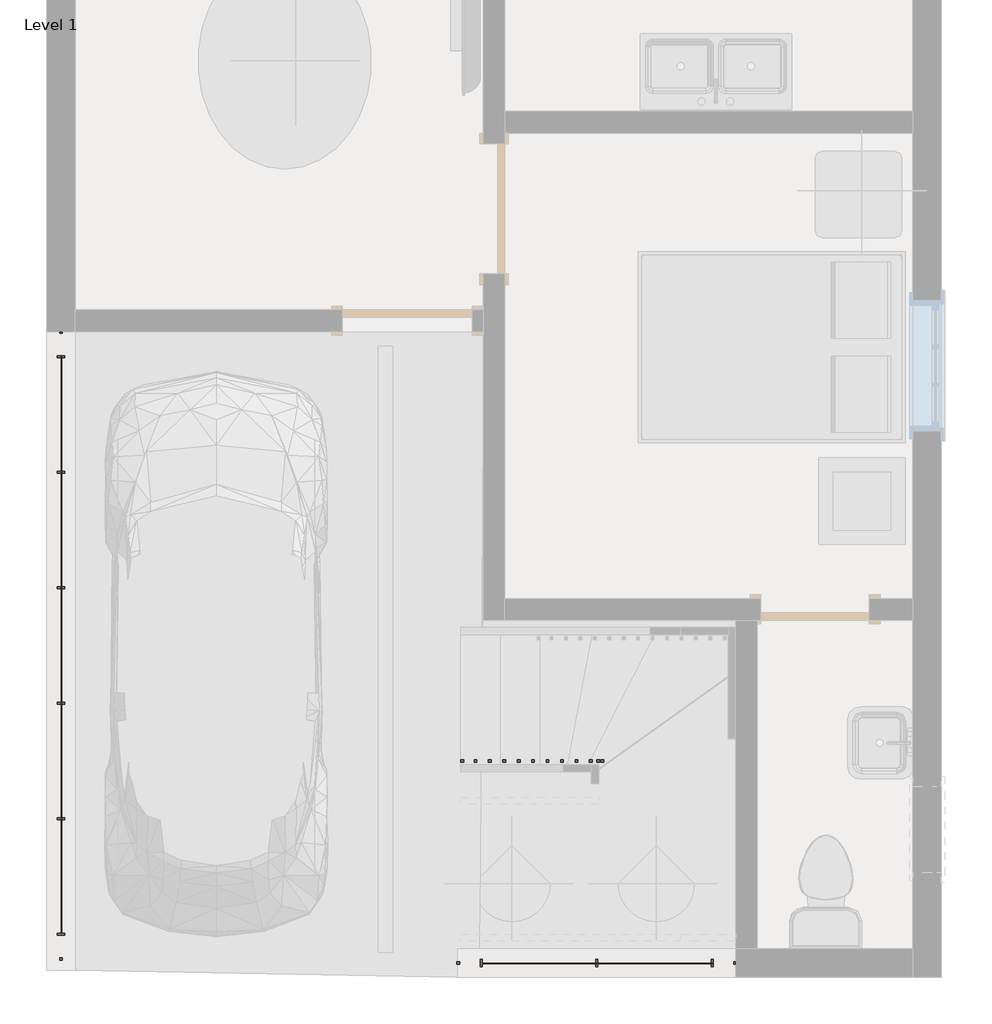
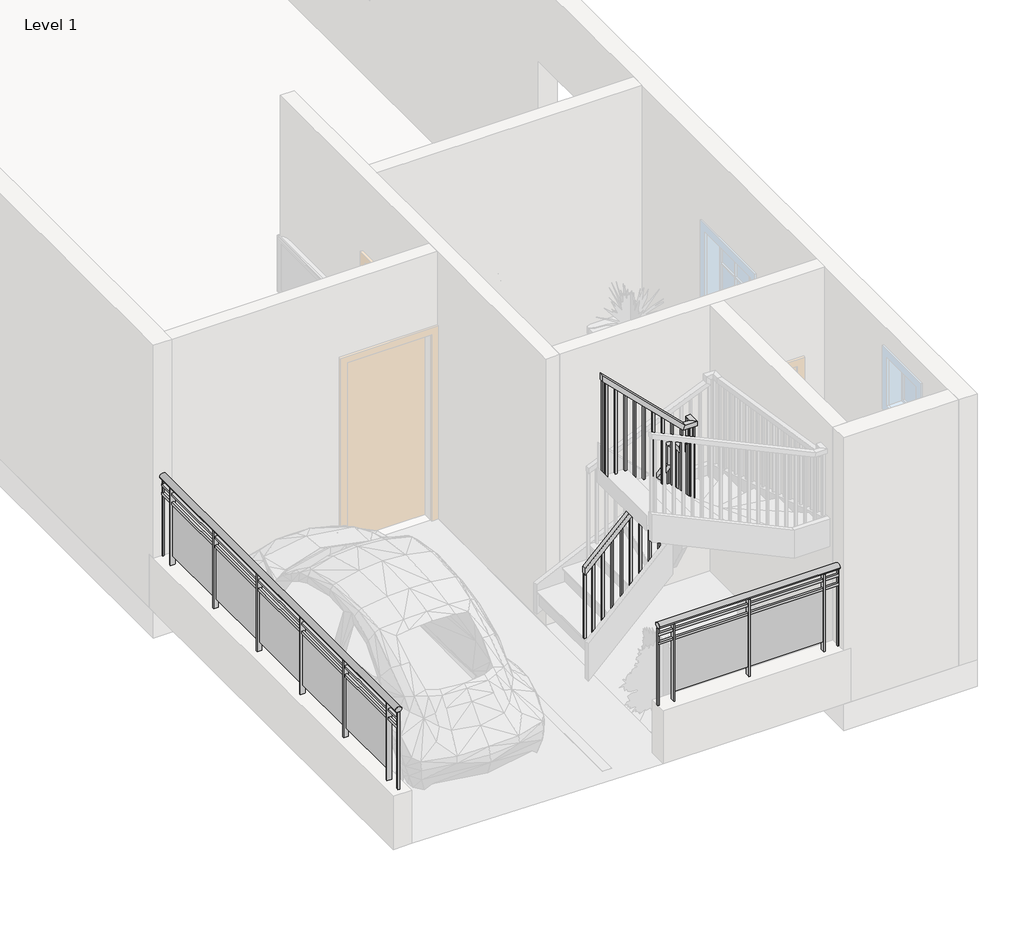
# One storey, part 2 of 3: 3 railings.
"""IFC4 building model written with IfcOpenShell, lengths in millimetres."""

from ifc_helpers import new_model, si_unit, point, frame, origin, place, context, project, spatial, polyline, ellipse_curve, trimmed, outline, extrude, faceted_brep, element, save
from ifc_brep_helpers import plane_surface, extruded_surface, advanced_brep

model = new_model("IFC4")

# Units and contexts
model_context = context("Model", 3, world=origin())
ifc_project = project(units=[si_unit("LENGTHUNIT", "METRE", prefix="MILLI")], contexts=[model_context])

# Site, building, storey
site = spatial("IfcSite", under=ifc_project)
building = spatial("IfcBuilding", under=site)
storey = spatial("IfcBuildingStorey", under=building, Name="Level 1", Elevation=0.0)

# Railings
placement = place(None, origin())
element("IfcRailing", 1, ObjectType="Glass Panel - Bottom Fill", at=placement, inside=storey, context=model_context, shape_type="SolidModel", body=[
    advanced_brep(
    [(-14578.2112155, 1512.0104001, 1524.0), (-14654.4112155, 1512.0104001, 1524.0), (-14578.2112155, -2907.5895999, 1524.0), (-14654.4112155, -2907.5895999, 1524.0)],
    [
        (0, 1, ellipse_curve(frame((-14616.3112155, 1512.0104001, 1524.0), z_axis=(0.0, 1.0, 0.0), x_axis=(-1.0, 0.0, 0.0)), 38.1, 28.575)),
        (1, 0, ellipse_curve(frame((-14616.3112155, 1512.0104001, 1524.0), z_axis=(0.0, 1.0, 0.0), x_axis=(-1.0, 0.0, 0.0)), 38.1, 28.575)),
        (2, 3, ellipse_curve(frame((-14616.3112155, -2907.5895999, 1524.0), z_axis=(0.0, -1.0, 0.0), x_axis=(-1.0, 0.0, 0.0)), 38.1, 28.575)),
        (3, 2, ellipse_curve(frame((-14616.3112155, -2907.5895999, 1524.0), z_axis=(0.0, -1.0, 0.0), x_axis=(-1.0, 0.0, 0.0)), 38.1, 28.575)),
        (0, 2),
        (3, 1),
    ],
    [
        plane_surface(frame((-14616.3112155, 1512.0104001, 1524.0), z_axis=(0.0, 1.0, 0.0), x_axis=(0.0, 0.0, -1.0))),
        plane_surface(frame((-14616.3112155, -2907.5895999, 1524.0), z_axis=(0.0, -1.0, 0.0), x_axis=(0.0, 0.0, -1.0))),
        extruded_surface(trimmed(ellipse_curve(frame((-14616.3112155, -2907.5895999, 1524.0), z_axis=(0.0, 1.0, 0.0), x_axis=(-1.0, 0.0, 0.0)), 38.1, 28.575), [point((-14578.2112155, -2907.5895999, 1524.0))], [point((-14654.4112155, -2907.5895999, 1524.0))], True, "CARTESIAN"), (0.0, 4419.6, 0.0), 4419.6),
        extruded_surface(trimmed(ellipse_curve(frame((-14616.3112155, -2907.5895999, 1524.0), z_axis=(0.0, 1.0, 0.0), x_axis=(-1.0, 0.0, 0.0)), 38.1, 28.575), [point((-14654.4112155, -2907.5895999, 1524.0))], [point((-14578.2112155, -2907.5895999, 1524.0))], True, "CARTESIAN"), (0.0, 4419.6, 0.0), 4419.6),
    ],
    [
        (0, [[1, 2]]),
        (1, [[3, 4]]),
        (2, [[-1, 5, -4, 6]]),
        (3, [[-2, -6, -3, -5]]),
    ],
),
    extrude(outline(polyline([(-14629.0112155, 1512.0104001), (-14603.6112155, 1512.0104001), (-14603.6112155, -2907.5895999), (-14629.0112155, -2907.5895999), (-14629.0112155, 1512.0104001)])), frame((0.0, 0.0, 1409.7), z_axis=(0.0, 0.0, 1.0), x_axis=(1.0, 0.0, 0.0)), (0.0, 0.0, 1.0), 25.4),
    extrude(outline(polyline([(-14629.0112155, 1512.0104001), (-14603.6112155, 1512.0104001), (-14603.6112155, -2907.5895999), (-14629.0112155, -2907.5895999), (-14629.0112155, 1512.0104001)])), frame((0.0, 0.0, 1308.1), z_axis=(0.0, 0.0, 1.0), x_axis=(1.0, 0.0, 0.0)), (0.0, 0.0, 1.0), 25.4),
    extrude(outline(polyline([(-14641.7112155, -2723.4395999), (-14590.9112155, -2723.4395999), (-14590.9112155, -2736.1395999), (-14641.7112155, -2736.1395999), (-14641.7112155, -2723.4395999)])), frame((0.0, 0.0, 609.6), z_axis=(0.0, 0.0, 1.0), x_axis=(1.0, 0.0, 0.0)), (0.0, 0.0, 1.0), 885.6788223),
    extrude(outline(polyline([(-14609.7760585, -1916.9895999), (-14609.7760585, -2729.7895999), (-14616.1260585, -2729.7895999), (-14616.1260585, -1916.9895999), (-14609.7760585, -1916.9895999)])), frame((0.0, 0.0, 711.2), z_axis=(0.0, 0.0, 1.0), x_axis=(1.0, 0.0, 0.0)), (0.0, 0.0, 1.0), 596.9),
    extrude(outline(polyline([(-14641.7112155, -1910.6395999), (-14590.9112155, -1910.6395999), (-14590.9112155, -1923.3395999), (-14641.7112155, -1923.3395999), (-14641.7112155, -1910.6395999)])), frame((0.0, 0.0, 609.6), z_axis=(0.0, 0.0, 1.0), x_axis=(1.0, 0.0, 0.0)), (0.0, 0.0, 1.0), 885.6788223),
    extrude(outline(polyline([(-14609.7760585, -1104.1895999), (-14609.7760585, -1916.9895999), (-14616.1260585, -1916.9895999), (-14616.1260585, -1104.1895999), (-14609.7760585, -1104.1895999)])), frame((0.0, 0.0, 711.2), z_axis=(0.0, 0.0, 1.0), x_axis=(1.0, 0.0, 0.0)), (0.0, 0.0, 1.0), 596.9),
    extrude(outline(polyline([(-14641.7112155, -1097.8395999), (-14590.9112155, -1097.8395999), (-14590.9112155, -1110.5395999), (-14641.7112155, -1110.5395999), (-14641.7112155, -1097.8395999)])), frame((0.0, 0.0, 609.6), z_axis=(0.0, 0.0, 1.0), x_axis=(1.0, 0.0, 0.0)), (0.0, 0.0, 1.0), 885.6788223),
    extrude(outline(polyline([(-14609.7760585, -291.3895999), (-14609.7760585, -1104.1895999), (-14616.1260585, -1104.1895999), (-14616.1260585, -291.3895999), (-14609.7760585, -291.3895999)])), frame((0.0, 0.0, 711.2), z_axis=(0.0, 0.0, 1.0), x_axis=(1.0, 0.0, 0.0)), (0.0, 0.0, 1.0), 596.9),
    extrude(outline(polyline([(-14641.7112155, -285.0395999), (-14590.9112155, -285.0395999), (-14590.9112155, -297.7395999), (-14641.7112155, -297.7395999), (-14641.7112155, -285.0395999)])), frame((0.0, 0.0, 609.6), z_axis=(0.0, 0.0, 1.0), x_axis=(1.0, 0.0, 0.0)), (0.0, 0.0, 1.0), 885.6788223),
    extrude(outline(polyline([(-14609.7760585, 521.4104001), (-14609.7760585, -291.3895999), (-14616.1260585, -291.3895999), (-14616.1260585, 521.4104001), (-14609.7760585, 521.4104001)])), frame((0.0, 0.0, 711.2), z_axis=(0.0, 0.0, 1.0), x_axis=(1.0, 0.0, 0.0)), (0.0, 0.0, 1.0), 596.9),
    extrude(outline(polyline([(-14641.7112155, 527.7604001), (-14590.9112155, 527.7604001), (-14590.9112155, 515.0604001), (-14641.7112155, 515.0604001), (-14641.7112155, 527.7604001)])), frame((0.0, 0.0, 609.6), z_axis=(0.0, 0.0, 1.0), x_axis=(1.0, 0.0, 0.0)), (0.0, 0.0, 1.0), 885.6788223),
    extrude(outline(polyline([(-14609.7760585, 1334.2104001), (-14609.7760585, 521.4104001), (-14616.1260585, 521.4104001), (-14616.1260585, 1334.2104001), (-14609.7760585, 1334.2104001)])), frame((0.0, 0.0, 711.2), z_axis=(0.0, 0.0, 1.0), x_axis=(1.0, 0.0, 0.0)), (0.0, 0.0, 1.0), 596.9),
    extrude(outline(polyline([(-14641.7112155, 1340.5604001), (-14590.9112155, 1340.5604001), (-14590.9112155, 1327.8604001), (-14641.7112155, 1327.8604001), (-14641.7112155, 1340.5604001)])), frame((0.0, 0.0, 609.6), z_axis=(0.0, 0.0, 1.0), x_axis=(1.0, 0.0, 0.0)), (0.0, 0.0, 1.0), 885.6788223),
    extrude(outline(polyline([(-14625.8362155, -2894.8895999), (-14606.7862155, -2894.8895999), (-14606.7862155, -2913.9395999), (-14625.8362155, -2913.9395999), (-14625.8362155, -2894.8895999)])), frame((0.0, 0.0, 609.6), z_axis=(0.0, 0.0, 1.0), x_axis=(1.0, 0.0, 0.0)), (0.0, 0.0, 1.0), 885.6788223),
    extrude(outline(polyline([(-14625.8362155, 1518.3604001), (-14606.7862155, 1518.3604001), (-14606.7862155, 1499.3104001), (-14625.8362155, 1499.3104001), (-14625.8362155, 1518.3604001)])), frame((0.0, 0.0, 609.6), z_axis=(0.0, 0.0, 1.0), x_axis=(1.0, 0.0, 0.0)), (0.0, 0.0, 1.0), 885.6788223),
])
element("IfcRailing", 2, ObjectType="Glass Panel - Bottom Fill", at=placement, inside=storey, context=model_context, shape_type="SolidModel", body=[
    advanced_brep(
    [(-9866.5112155, -2971.0895999, 1524.0), (-9866.5112155, -2894.8895999, 1524.0), (-11822.3112155, -2971.0895999, 1524.0), (-11822.3112155, -2894.8895999, 1524.0)],
    [
        (0, 1, ellipse_curve(frame((-9866.5112155, -2932.9895999, 1524.0), z_axis=(1.0, 0.0, 0.0), x_axis=(0.0, 1.0, 0.0)), 38.1, 28.575)),
        (1, 0, ellipse_curve(frame((-9866.5112155, -2932.9895999, 1524.0), z_axis=(1.0, 0.0, 0.0), x_axis=(0.0, 1.0, 0.0)), 38.1, 28.575)),
        (2, 3, ellipse_curve(frame((-11822.3112155, -2932.9895999, 1524.0), z_axis=(-1.0, 0.0, 0.0), x_axis=(0.0, 1.0, 0.0)), 38.1, 28.575)),
        (3, 2, ellipse_curve(frame((-11822.3112155, -2932.9895999, 1524.0), z_axis=(-1.0, 0.0, 0.0), x_axis=(0.0, 1.0, 0.0)), 38.1, 28.575)),
        (0, 2),
        (3, 1),
    ],
    [
        plane_surface(frame((-9866.5112155, -2932.9895999, 1524.0), z_axis=(1.0, 0.0, 0.0), x_axis=(0.0, -1.0, 0.0))),
        plane_surface(frame((-11822.3112155, -2932.9895999, 1524.0), z_axis=(-1.0, 0.0, 0.0), x_axis=(0.0, -1.0, 0.0))),
        extruded_surface(trimmed(ellipse_curve(frame((-11822.3112155, -2932.9895999, 1524.0), z_axis=(1.0, 0.0, 0.0), x_axis=(0.0, 1.0, 0.0)), 38.1, 28.575), [point((-11822.3112155, -2971.0895999, 1524.0))], [point((-11822.3112155, -2894.8895999, 1524.0))], True, "CARTESIAN"), (1955.7999999999993, 0.0, 0.0), 1955.7999999999993),
        extruded_surface(trimmed(ellipse_curve(frame((-11822.3112155, -2932.9895999, 1524.0), z_axis=(1.0, 0.0, 0.0), x_axis=(0.0, 1.0, 0.0)), 38.1, 28.575), [point((-11822.3112155, -2894.8895999, 1524.0))], [point((-11822.3112155, -2971.0895999, 1524.0))], True, "CARTESIAN"), (1955.7999999999993, 0.0, 0.0), 1955.7999999999993),
    ],
    [
        (0, [[1, 2]]),
        (1, [[3, 4]]),
        (2, [[-1, 5, -4, 6]]),
        (3, [[-2, -6, -3, -5]]),
    ],
),
    extrude(outline(polyline([(-9866.5112155, -2920.2895999), (-9866.5112155, -2945.6895999), (-11822.3112155, -2945.6895999), (-11822.3112155, -2920.2895999), (-9866.5112155, -2920.2895999)])), frame((0.0, 0.0, 1409.7), z_axis=(0.0, 0.0, 1.0), x_axis=(1.0, 0.0, 0.0)), (0.0, 0.0, 1.0), 25.4),
    extrude(outline(polyline([(-9866.5112155, -2920.2895999), (-9866.5112155, -2945.6895999), (-11822.3112155, -2945.6895999), (-11822.3112155, -2920.2895999), (-9866.5112155, -2920.2895999)])), frame((0.0, 0.0, 1308.1), z_axis=(0.0, 0.0, 1.0), x_axis=(1.0, 0.0, 0.0)), (0.0, 0.0, 1.0), 25.4),
    extrude(outline(polyline([(-11650.8612155, -2907.5895999), (-11650.8612155, -2958.3895999), (-11663.5612155, -2958.3895999), (-11663.5612155, -2907.5895999), (-11650.8612155, -2907.5895999)])), frame((0.0, 0.0, 609.6), z_axis=(0.0, 0.0, 1.0), x_axis=(1.0, 0.0, 0.0)), (0.0, 0.0, 1.0), 885.6788223),
    extrude(outline(polyline([(-10844.4112155, -2939.5247569), (-11657.2112155, -2939.5247569), (-11657.2112155, -2933.1747569), (-10844.4112155, -2933.1747569), (-10844.4112155, -2939.5247569)])), frame((0.0, 0.0, 711.2), z_axis=(0.0, 0.0, 1.0), x_axis=(1.0, 0.0, 0.0)), (0.0, 0.0, 1.0), 596.9),
    extrude(outline(polyline([(-10838.0612155, -2907.5895999), (-10838.0612155, -2958.3895999), (-10850.7612155, -2958.3895999), (-10850.7612155, -2907.5895999), (-10838.0612155, -2907.5895999)])), frame((0.0, 0.0, 609.6), z_axis=(0.0, 0.0, 1.0), x_axis=(1.0, 0.0, 0.0)), (0.0, 0.0, 1.0), 885.6788223),
    extrude(outline(polyline([(-10031.6112155, -2939.5247569), (-10844.4112155, -2939.5247569), (-10844.4112155, -2933.1747569), (-10031.6112155, -2933.1747569), (-10031.6112155, -2939.5247569)])), frame((0.0, 0.0, 711.2), z_axis=(0.0, 0.0, 1.0), x_axis=(1.0, 0.0, 0.0)), (0.0, 0.0, 1.0), 596.9),
    extrude(outline(polyline([(-10025.2612155, -2907.5895999), (-10025.2612155, -2958.3895999), (-10037.9612155, -2958.3895999), (-10037.9612155, -2907.5895999), (-10025.2612155, -2907.5895999)])), frame((0.0, 0.0, 609.6), z_axis=(0.0, 0.0, 1.0), x_axis=(1.0, 0.0, 0.0)), (0.0, 0.0, 1.0), 885.6788223),
    extrude(outline(polyline([(-11809.6112155, -2923.4645999), (-11809.6112155, -2942.5145999), (-11828.6612155, -2942.5145999), (-11828.6612155, -2923.4645999), (-11809.6112155, -2923.4645999)])), frame((0.0, 0.0, 609.6), z_axis=(0.0, 0.0, 1.0), x_axis=(1.0, 0.0, 0.0)), (0.0, 0.0, 1.0), 885.6788223),
    extrude(outline(polyline([(-9860.1612155, -2923.4645999), (-9860.1612155, -2942.5145999), (-9879.2112155, -2942.5145999), (-9879.2112155, -2923.4645999), (-9860.1612155, -2923.4645999)])), frame((0.0, 0.0, 609.6), z_axis=(0.0, 0.0, 1.0), x_axis=(1.0, 0.0, 0.0)), (0.0, 0.0, 1.0), 885.6788223),
])
element("IfcRailing", 3, ObjectType="Handrail - Rectangular", at=placement, inside=storey, context=model_context, shape_type="SolidModel", body=[
    faceted_brep([(-11800.6429074, -1485.1895999, 1316.3704569), (-11800.6429074, -1485.1895999, 1245.0455517), (-11800.6429074, -1535.9895999, 1245.0455517), (-11800.6429074, -1535.9895999, 1316.3704569), (-10907.9112155, -1485.1895999, 2196.2028354), (-10857.1112155, -1485.1895999, 2174.9439077), (-10857.1112155, -1535.9895999, 2174.9439077), (-10907.9112155, -1535.9895999, 2196.2028354), (-10907.9112155, -1485.1895999, 2414.6281882), (-10857.1112155, -1485.1895999, 2363.8281882), (-10857.1112155, -1535.9895999, 2363.8281882), (-10907.9112155, -1535.9895999, 2414.6281882), (-10780.9112155, -1485.1895999, 2414.6281882), (-10780.9112155, -1485.1895999, 2363.8281882), (-10831.7112155, -1535.9895999, 2363.8281882), (-10831.7112155, -1535.9895999, 2414.6281882), (-10780.9112155, -1612.1895999, 2414.6281882), (-10780.9112155, -1641.3109337, 2363.8281882), (-10831.7112155, -1641.3109337, 2363.8281882), (-10831.7112155, -1612.1895999, 2414.6281882), (-10780.9112155, -1739.1895999, 2631.5051451), (-10780.9112155, -1789.9895999, 2617.7256424), (-10831.7112155, -1789.9895999, 2617.7256424), (-10831.7112155, -1739.1895999, 2631.5051451), (-10780.9112155, -1739.1895999, 2849.930498), (-10780.9112155, -1789.9895999, 2799.130498), (-10831.7112155, -1789.9895999, 2799.130498), (-10831.7112155, -1739.1895999, 2849.930498), (-10780.9112155, -1866.1895999, 2849.930498), (-10780.9112155, -1866.1895999, 2799.130498), (-10831.7112155, -1815.3895999, 2799.130498), (-10831.7112155, -1815.3895999, 2849.930498), (-10907.9112155, -1866.1895999, 2849.930498), (-10928.7370385, -1866.1895999, 2799.130498), (-10928.7370385, -1815.3895999, 2799.130498), (-10907.9112155, -1815.3895999, 2849.930498), (-11800.6429074, -1866.1895999, 3729.7628764), (-11800.6429074, -1815.3895999, 3729.7628764), (-11800.6429074, -1815.3895999, 3658.4379712), (-11800.6429074, -1866.1895999, 3658.4379712)], [[[0, 1, 2, 3]], [[1, 0, 4, 5]], [[2, 1, 5, 6]], [[3, 2, 6, 7]], [[0, 3, 7, 4]], [[5, 4, 8, 9]], [[6, 5, 9, 10]], [[7, 6, 10, 11]], [[4, 7, 11, 8]], [[9, 8, 12, 13]], [[10, 9, 13, 14]], [[11, 10, 14, 15]], [[8, 11, 15, 12]], [[13, 12, 16, 17]], [[14, 13, 17, 18]], [[15, 14, 18, 19]], [[12, 15, 19, 16]], [[17, 16, 20, 21]], [[18, 17, 21, 22]], [[19, 18, 22, 23]], [[16, 19, 23, 20]], [[21, 20, 24, 25]], [[22, 21, 25, 26]], [[23, 22, 26, 27]], [[20, 23, 27, 24]], [[25, 24, 28, 29]], [[26, 25, 29, 30]], [[27, 26, 30, 31]], [[24, 27, 31, 28]], [[29, 28, 32, 33]], [[30, 29, 33, 34]], [[31, 30, 34, 35]], [[28, 31, 35, 32]], [[36, 37, 38, 39]], [[33, 32, 36, 39]], [[34, 33, 39, 38]], [[35, 34, 38, 37]], [[32, 35, 37, 36]]]),
    extrude(outline(polyline([(3597.8779463, -11739.1950058), (3616.6526879, -11758.2450058), (2540.0, -11758.2450058), (2540.0, -11739.1950058), (3597.8779463, -11739.1950058)])), frame((0.0, -1850.3145999, 0.0), z_axis=(0.0, 1.0, 0.0), x_axis=(0.0, 0.0, 1.0)), (0.0, 0.0, 1.0), 19.05),
    extrude(outline(polyline([(3497.7459913, -11637.5950058), (3516.5207329, -11656.6450058), (2540.0, -11656.6450058), (2540.0, -11637.5950058), (3497.7459913, -11637.5950058)])), frame((0.0, -1850.3145999, 0.0), z_axis=(0.0, 1.0, 0.0), x_axis=(0.0, 0.0, 1.0)), (0.0, 0.0, 1.0), 19.05),
    extrude(outline(polyline([(3397.6140362, -11535.9950058), (3416.3887778, -11555.0450058), (2540.0, -11555.0450058), (2540.0, -11535.9950058), (3397.6140362, -11535.9950058)])), frame((0.0, -1850.3145999, 0.0), z_axis=(0.0, 1.0, 0.0), x_axis=(0.0, 0.0, 1.0)), (0.0, 0.0, 1.0), 19.05),
    extrude(outline(polyline([(3297.4820812, -11434.3950058), (3316.2568227, -11453.4450058), (2370.6666667, -11453.4450058), (2370.6666667, -11434.3950058), (3297.4820812, -11434.3950058)])), frame((0.0, -1850.3145999, 0.0), z_axis=(0.0, 1.0, 0.0), x_axis=(0.0, 0.0, 1.0)), (0.0, 0.0, 1.0), 19.05),
    extrude(outline(polyline([(3197.3501261, -11332.7950058), (3216.1248677, -11351.8450058), (2370.6666667, -11351.8450058), (2370.6666667, -11332.7950058), (3197.3501261, -11332.7950058)])), frame((0.0, -1850.3145999, 0.0), z_axis=(0.0, 1.0, 0.0), x_axis=(0.0, 0.0, 1.0)), (0.0, 0.0, 1.0), 19.05),
    extrude(outline(polyline([(3097.218171, -11231.1950058), (3115.9929126, -11250.2450058), (2201.3333333, -11250.2450058), (2201.3333333, -11231.1950058), (3097.218171, -11231.1950058)])), frame((0.0, -1850.3145999, 0.0), z_axis=(0.0, 1.0, 0.0), x_axis=(0.0, 0.0, 1.0)), (0.0, 0.0, 1.0), 19.05),
    extrude(outline(polyline([(2997.086216, -11129.5950058), (3015.8609575, -11148.6450058), (2201.3333333, -11148.6450058), (2201.3333333, -11129.5950058), (2997.086216, -11129.5950058)])), frame((0.0, -1850.3145999, 0.0), z_axis=(0.0, 1.0, 0.0), x_axis=(0.0, 0.0, 1.0)), (0.0, 0.0, 1.0), 19.05),
    extrude(outline(polyline([(2896.9542609, -11027.9950058), (2915.7290025, -11047.0450058), (2032.0, -11047.0450058), (2032.0, -11027.9950058), (2896.9542609, -11027.9950058)])), frame((0.0, -1850.3145999, 0.0), z_axis=(0.0, 1.0, 0.0), x_axis=(0.0, 0.0, 1.0)), (0.0, 0.0, 1.0), 19.05),
    extrude(outline(polyline([(2796.8223058, -10926.3950058), (2815.5970474, -10945.4450058), (2032.0, -10945.4450058), (2032.0, -10926.3950058), (2796.8223058, -10926.3950058)])), frame((0.0, -1850.3145999, 0.0), z_axis=(0.0, 1.0, 0.0), x_axis=(0.0, 0.0, 1.0)), (0.0, 0.0, 1.0), 19.05),
    extrude(outline(polyline([(-1739.479151, 2531.4693239), (-1720.429151, 2498.9377803), (-1720.429151, 1524.0), (-1739.479151, 1524.0), (-1739.479151, 2531.4693239)])), frame((-10815.8362155, 0.0, 0.0), z_axis=(1.0, 0.0, 0.0), x_axis=(0.0, 1.0, 0.0)), (0.0, 0.0, 1.0), 19.05),
    extrude(outline(polyline([(-1637.879151, 2357.9677583), (-1618.829151, 2325.4362148), (-1618.829151, 1524.0), (-1637.879151, 1524.0), (-1637.879151, 2357.9677583)])), frame((-10815.8362155, 0.0, 0.0), z_axis=(1.0, 0.0, 0.0), x_axis=(0.0, 1.0, 0.0)), (0.0, 0.0, 1.0), 19.05),
    extrude(outline(polyline([(2155.620518, -10876.7179074), (2136.8457765, -10895.7679074), (1185.3333333, -10895.7679074), (1185.3333333, -10876.7179074), (2155.620518, -10876.7179074)])), frame((0.0, -1520.1145999, 0.0), z_axis=(0.0, 1.0, 0.0), x_axis=(0.0, 0.0, 1.0)), (0.0, 0.0, 1.0), 19.05),
    extrude(outline(polyline([(2055.488563, -10978.3179074), (2036.7138214, -10997.3679074), (1016.0, -10997.3679074), (1016.0, -10978.3179074), (2055.488563, -10978.3179074)])), frame((0.0, -1520.1145999, 0.0), z_axis=(0.0, 1.0, 0.0), x_axis=(0.0, 0.0, 1.0)), (0.0, 0.0, 1.0), 19.05),
    extrude(outline(polyline([(1955.3566079, -11079.9179074), (1936.5818663, -11098.9679074), (846.6666667, -11098.9679074), (846.6666667, -11079.9179074), (1955.3566079, -11079.9179074)])), frame((0.0, -1520.1145999, 0.0), z_axis=(0.0, 1.0, 0.0), x_axis=(0.0, 0.0, 1.0)), (0.0, 0.0, 1.0), 19.05),
    extrude(outline(polyline([(1855.2246528, -11181.5179074), (1836.4499113, -11200.5679074), (846.6666667, -11200.5679074), (846.6666667, -11181.5179074), (1855.2246528, -11181.5179074)])), frame((0.0, -1520.1145999, 0.0), z_axis=(0.0, 1.0, 0.0), x_axis=(0.0, 0.0, 1.0)), (0.0, 0.0, 1.0), 19.05),
    extrude(outline(polyline([(1755.0926978, -11283.1179074), (1736.3179562, -11302.1679074), (677.3333333, -11302.1679074), (677.3333333, -11283.1179074), (1755.0926978, -11283.1179074)])), frame((0.0, -1520.1145999, 0.0), z_axis=(0.0, 1.0, 0.0), x_axis=(0.0, 0.0, 1.0)), (0.0, 0.0, 1.0), 19.05),
    extrude(outline(polyline([(1654.9607427, -11384.7179074), (1636.1860011, -11403.7679074), (677.3333333, -11403.7679074), (677.3333333, -11384.7179074), (1654.9607427, -11384.7179074)])), frame((0.0, -1520.1145999, 0.0), z_axis=(0.0, 1.0, 0.0), x_axis=(0.0, 0.0, 1.0)), (0.0, 0.0, 1.0), 19.05),
    extrude(outline(polyline([(1554.8287877, -11486.3179074), (1536.0540461, -11505.3679074), (677.3333333, -11505.3679074), (677.3333333, -11486.3179074), (1554.8287877, -11486.3179074)])), frame((0.0, -1520.1145999, 0.0), z_axis=(0.0, 1.0, 0.0), x_axis=(0.0, 0.0, 1.0)), (0.0, 0.0, 1.0), 19.05),
    extrude(outline(polyline([(1454.6968326, -11587.9179074), (1435.922091, -11606.9679074), (508.0, -11606.9679074), (508.0, -11587.9179074), (1454.6968326, -11587.9179074)])), frame((0.0, -1520.1145999, 0.0), z_axis=(0.0, 1.0, 0.0), x_axis=(0.0, 0.0, 1.0)), (0.0, 0.0, 1.0), 19.05),
    extrude(outline(polyline([(1354.5648775, -11689.5179074), (1335.790136, -11708.5679074), (508.0, -11708.5679074), (508.0, -11689.5179074), (1354.5648775, -11689.5179074)])), frame((0.0, -1520.1145999, 0.0), z_axis=(0.0, 1.0, 0.0), x_axis=(0.0, 0.0, 1.0)), (0.0, 0.0, 1.0), 19.05),
    extrude(outline(polyline([(-10824.7950058, -1831.2645999), (-10824.7950058, -1850.3145999), (-10843.8450058, -1850.3145999), (-10843.8450058, -1831.2645999), (-10824.7950058, -1831.2645999)])), frame((0.0, 0.0, 1862.6666667), z_axis=(0.0, 0.0, 1.0), x_axis=(1.0, 0.0, 0.0)), (0.0, 0.0, 1.0), 936.4638313),
    extrude(outline(polyline([(-10815.8362155, -1831.2645999), (-10796.7862155, -1831.2645999), (-10796.7862155, -1850.3145999), (-10815.8362155, -1850.3145999), (-10815.8362155, -1831.2645999)])), frame((0.0, 0.0, 1862.6666667), z_axis=(0.0, 0.0, 1.0), x_axis=(1.0, 0.0, 0.0)), (0.0, 0.0, 1.0), 936.4638313),
    extrude(outline(polyline([(-10815.8362155, -1815.1000488), (-10796.7862155, -1815.1000488), (-10796.7862155, -1834.1500488), (-10815.8362155, -1834.1500488), (-10815.8362155, -1815.1000488)])), frame((0.0, 0.0, 1693.3333333), z_axis=(0.0, 0.0, 1.0), x_axis=(1.0, 0.0, 0.0)), (0.0, 0.0, 1.0), 1105.7971646),
    extrude(outline(polyline([(-10815.8362155, -1517.229151), (-10796.7862155, -1517.229151), (-10796.7862155, -1536.279151), (-10815.8362155, -1536.279151), (-10815.8362155, -1517.229151)])), frame((0.0, 0.0, 1354.6666667), z_axis=(0.0, 0.0, 1.0), x_axis=(1.0, 0.0, 0.0)), (0.0, 0.0, 1.0), 1009.1615215),
    extrude(outline(polyline([(-10815.8362155, -1520.1145999), (-10815.8362155, -1501.0645999), (-10796.7862155, -1501.0645999), (-10796.7862155, -1520.1145999), (-10815.8362155, -1520.1145999)])), frame((0.0, 0.0, 1185.3333333), z_axis=(0.0, 0.0, 1.0), x_axis=(1.0, 0.0, 0.0)), (0.0, 0.0, 1.0), 1178.4948549),
    extrude(outline(polyline([(-10843.8450058, -1520.1145999), (-10843.8450058, -1501.0645999), (-10824.7950058, -1501.0645999), (-10824.7950058, -1520.1145999), (-10843.8450058, -1520.1145999)])), frame((0.0, 0.0, 1185.3333333), z_axis=(0.0, 0.0, 1.0), x_axis=(1.0, 0.0, 0.0)), (0.0, 0.0, 1.0), 1178.4948549),
    extrude(outline(polyline([(3639.6632296, -11781.5929074), (3658.4379712, -11800.6429074), (2540.0, -11800.6429074), (2540.0, -11781.5929074), (3639.6632296, -11781.5929074)])), frame((0.0, -1850.3145999, 0.0), z_axis=(0.0, 1.0, 0.0), x_axis=(0.0, 0.0, 1.0)), (0.0, 0.0, 1.0), 19.05),
    extrude(outline(polyline([(1263.8202933, -11781.5929074), (1245.0455517, -11800.6429074), (508.0, -11800.6429074), (508.0, -11781.5929074), (1263.8202933, -11781.5929074)])), frame((0.0, -1520.1145999, 0.0), z_axis=(0.0, 1.0, 0.0), x_axis=(0.0, 0.0, 1.0)), (0.0, 0.0, 1.0), 19.05),
])

save(model, "model.ifc")

# Revit data of these elements
# Type "Glass Panel - Bottom Fill"
#   Assembly Code = "C2010400"
#   built-in parameter 1008612 = 0.0416667 (stored number, unit not read)
#   built-in parameter 1008611 = 0.0416667 (stored number, unit not read)
#   built-in parameter 1008609 = 0.333333 (stored number, unit not read)
#   built-in parameter 1008604 = 0.166667 (stored number, unit not read)
#   built-in parameter 1008603 = 0.166667 (stored number, unit not read)
#   Railing Height = 3' - 0"
#   built-in parameter 1008630 = 2
#   built-in parameter 1008610 = 2
#   built-in parameter 1008618 = Baluster - Square : 3/4"
# Type "Handrail - Rectangular"
#   Assembly Code = "C2010400"
#   built-in parameter 1008612 = 0.0416667 (stored number, unit not read)
#   built-in parameter 1008611 = 0.0416667 (stored number, unit not read)
#   built-in parameter 1008609 = 0.333333 (stored number, unit not read)
#   built-in parameter 1008604 = 0.166667 (stored number, unit not read)
#   built-in parameter 1008603 = 0.166667 (stored number, unit not read)
#   Railing Height = 3' - 0"
#   built-in parameter 1008630 = 2
#   built-in parameter 1008610 = 2
#   built-in parameter 1008618 = Baluster - Square : 3/4"
# Elements 1, 2 (IfcRailing, "Glass Panel - Bottom Fill")
#   built-in parameter 1008621 = 2 (stored number, unit not read)
#   Phase Created = New Construction
#   Materials on its faces: "Glass"
# Element 3 (IfcRailing, "Handrail - Rectangular")
#   Phase Created = New Construction
# Materials
#   "Glass": class "Glass", colour RGB 0 128 192, transparency 0.75, Description = "Soda Lime Glass", Cost = 0
